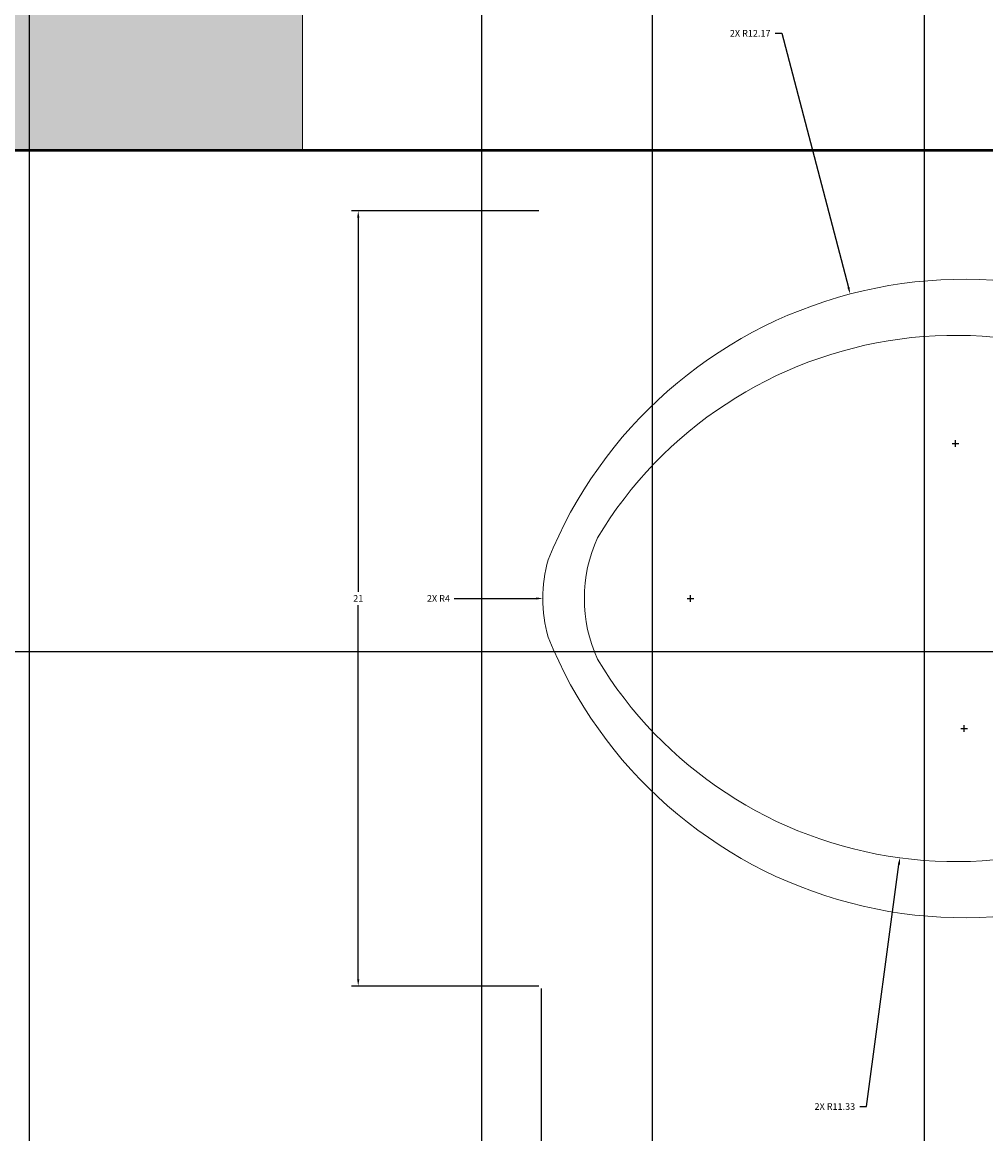
# Model space of a CAD drawing. Units: inches. Extents: x 2231 to 2461, y 2045 to 2455.
# Tile 90 of 95: x 2384 to 2410, y 2400 to 2430. Entities that reach past the tile are written whole.
import ezdxf

# ---------------------------------------------------------------- set-up
doc = ezdxf.new("R2010")
doc.units = ezdxf.units.IN
for name, color, linetype, lineweight in [('A-ANNO-DIMS', 2, 'Continuous', 18), ('A-FLOR-FIXT', 9, 'Continuous', 18), ('A-GLAZ', 4, 'Continuous', 18), ('A-WALL', 7, 'Continuous', 50)]:
    doc.layers.add(name, color=color, linetype=linetype, lineweight=lineweight)
doc.layers.add('A-WALL-PATT', color=18, linetype='Continuous', lineweight=13, true_color=0x000000)
doc.styles.get("Standard").update_dxf_attribs({"font": 'arial.ttf'})
doc.dimstyles.get("Standard").update_dxf_attribs({"dimtxt": 0.18, "dimasz": 0.18, "dimexe": 0.18, "dimexo": 0.0625, "dimgap": 0.09, "dimtad": 0, "dimtih": 1, "dimtoh": 1, "dimdec": 4, "dimzin": 0, "dimdsep": 46, "dimtxsty": 'Standard', "dimcen": 0.09, "dimadec": 0, "dimazin": 0, "dimtfac": 1, "dimtdec": 4, "dimtofl": 0, "dimtmove": 0, "dimatfit": 3, "dimfxl": 1, "dimtolj": 1, "dimtzin": 0, "dimarcsym": 0})

# ---------------------------------------------------------------- blocks, each defined once
blk = doc.blocks.new('Toilet - top')
for centre, radius, start, end in [((3.52, -21.58), 12.169, 141.4691, 247.9714), ((4.2, -21.817), 11.329, 136.3677, 238.9468), ((-3.519, -21.58), 12.169, 292.0284, 38.5307), ((-4.2, -21.817), 11.329, 301.053, 43.6321), ((0, -27.876), 4, 245.7318, 294.2682), ((0, -29), 4, 254.8605, 285.1395)]:
    blk.add_arc(centre, radius, start, end)
blk = doc.blocks.new('*D21')
at = {"layer": 'A-ANNO-DIMS', "color": 0, "lineweight": -2, "transparency": 16777216}
for p, q in [((2398.404, 2404.126), (2398.404, 2399.052)), ((2431.45, 2404.126), (2431.45, 2399.052)), ((2398.584, 2399.232), (2414.46, 2399.232)), ((2431.27, 2399.232), (2415.394, 2399.232))]:
    blk.add_line(p, q, dxfattribs=at)
at = {"layer": 'A-ANNO-DIMS', "color": 0, "transparency": 16777216}
for points in [[(2398.584, 2399.262), (2398.584, 2399.202), (2398.404, 2399.232)], [(2431.27, 2399.262), (2431.27, 2399.202), (2431.45, 2399.232)]]:
    blk.add_solid(points, dxfattribs=at)
at = {"layer": 'Defpoints', "color": 0, "transparency": 16777216}
for p in [(2398.404, 2404.189), (2431.45, 2404.189), (2431.45, 2399.232)]:
    blk.add_point(p, dxfattribs=at)
at = {"layer": 'A-ANNO-DIMS', "color": 0, "transparency": 16777216, "insert": (2414.927, 2399.232), "char_height": 0.18, "attachment_point": 5}
blk.add_mtext('\\A1;WC 33', dxfattribs=at)
blk = doc.blocks.new('*D22')
at = {"layer": 'A-ANNO-DIMS', "color": 0, "lineweight": -2, "transparency": 16777216}
for p, q in [((2398.342, 2425.189), (2393.267, 2425.189)), ((2393.447, 2425.009), (2393.447, 2414.869)), ((2393.447, 2404.369), (2393.447, 2414.508)), ((2398.342, 2404.189), (2393.267, 2404.189))]:
    blk.add_line(p, q, dxfattribs=at)
at = {"layer": 'A-ANNO-DIMS', "color": 0, "transparency": 16777216}
for points in [[(2393.417, 2425.009), (2393.477, 2425.009), (2393.447, 2425.189)], [(2393.417, 2404.369), (2393.477, 2404.369), (2393.447, 2404.189)]]:
    blk.add_solid(points, dxfattribs=at)
at = {"layer": 'Defpoints', "color": 0, "transparency": 16777216}
for p in [(2398.404, 2425.189), (2393.447, 2404.189), (2398.404, 2404.189)]:
    blk.add_point(p, dxfattribs=at)
at = {"layer": 'A-ANNO-DIMS', "color": 0, "transparency": 16777216, "insert": (2393.447, 2414.689), "char_height": 0.18, "attachment_point": 5}
blk.add_mtext('\\A1;21', dxfattribs=at)
blk = doc.blocks.new('*D36')
at = {"layer": 'A-ANNO-DIMS', "color": 0, "lineweight": -2, "transparency": 16777216}
for p, q in [((2372.794, 2426.895), (2372.794, 2454.645)), ((2372.974, 2454.465), (2402.574, 2454.465)), ((2432.614, 2454.465), (2403.013, 2454.465)), ((2432.794, 2426.895), (2432.794, 2454.645))]:
    blk.add_line(p, q, dxfattribs=at)
at = {"layer": 'A-ANNO-DIMS', "color": 0, "transparency": 16777216}
for points in [[(2372.974, 2454.495), (2372.974, 2454.435), (2372.794, 2454.465)], [(2432.614, 2454.495), (2432.614, 2454.435), (2432.794, 2454.465)]]:
    blk.add_solid(points, dxfattribs=at)
at = {"layer": 'Defpoints', "color": 0, "transparency": 16777216}
for p in [(2432.794, 2454.465), (2372.794, 2426.833), (2432.794, 2426.833)]:
    blk.add_point(p, dxfattribs=at)
at = {"layer": 'A-ANNO-DIMS', "color": 0, "transparency": 16777216, "insert": (2402.794, 2454.465), "char_height": 0.18, "attachment_point": 5}
blk.add_mtext('\\A1;60', dxfattribs=at)
blk = doc.blocks.new('*D42')
at = {"layer": 'A-ANNO-DIMS', "color": 0, "lineweight": -2, "transparency": 16777216}
for p, q in [((2396.794, 2286.895), (2396.794, 2454.645)), ((2396.974, 2454.465), (2414.575, 2454.465)), ((2432.614, 2454.465), (2415.012, 2454.465)), ((2432.794, 2286.895), (2432.794, 2454.645))]:
    blk.add_line(p, q, dxfattribs=at)
at = {"layer": 'A-ANNO-DIMS', "color": 0, "transparency": 16777216}
for points in [[(2396.974, 2454.495), (2396.974, 2454.435), (2396.794, 2454.465)], [(2432.614, 2454.495), (2432.614, 2454.435), (2432.794, 2454.465)]]:
    blk.add_solid(points, dxfattribs=at)
at = {"layer": 'Defpoints', "color": 0, "transparency": 16777216}
for p in [(2432.794, 2454.465), (2396.794, 2286.833), (2432.794, 2286.833)]:
    blk.add_point(p, dxfattribs=at)
at = {"layer": 'A-ANNO-DIMS', "color": 0, "transparency": 16777216, "insert": (2414.794, 2454.465), "char_height": 0.18, "attachment_point": 5}
blk.add_mtext('\\A1;36', dxfattribs=at)
blk = doc.blocks.new('*D59')
at = {"layer": 'A-ANNO-DIMS', "color": 0, "lineweight": -2, "transparency": 16777216}
for p, q in [((2408.794, 2182.895), (2408.794, 2454.645)), ((2408.974, 2454.465), (2420.573, 2454.465)), ((2432.614, 2454.465), (2421.014, 2454.465)), ((2432.794, 2182.895), (2432.794, 2454.645))]:
    blk.add_line(p, q, dxfattribs=at)
at = {"layer": 'A-ANNO-DIMS', "color": 0, "transparency": 16777216}
for points in [[(2408.974, 2454.495), (2408.974, 2454.435), (2408.794, 2454.465)], [(2432.614, 2454.495), (2432.614, 2454.435), (2432.794, 2454.465)]]:
    blk.add_solid(points, dxfattribs=at)
at = {"layer": 'Defpoints', "color": 0, "transparency": 16777216}
for p in [(2432.794, 2454.465), (2408.794, 2182.833), (2432.794, 2182.833)]:
    blk.add_point(p, dxfattribs=at)
at = {"layer": 'A-ANNO-DIMS', "color": 0, "transparency": 16777216, "insert": (2420.794, 2454.465), "char_height": 0.18, "attachment_point": 5}
blk.add_mtext('\\A1;24', dxfattribs=at)
blk = doc.blocks.new('*D66')
at = {"layer": 'A-ANNO-DIMS', "color": 0, "lineweight": -2, "transparency": 16777216}
for p, q in [((2348.189, 2096.895), (2348.189, 2454.645)), ((2348.369, 2454.465), (2378.167, 2454.465)), ((2408.614, 2454.465), (2378.815, 2454.465)), ((2408.794, 2096.895), (2408.794, 2454.645))]:
    blk.add_line(p, q, dxfattribs=at)
at = {"layer": 'A-ANNO-DIMS', "color": 0, "transparency": 16777216}
for points in [[(2348.369, 2454.495), (2348.369, 2454.435), (2348.189, 2454.465)], [(2408.614, 2454.495), (2408.614, 2454.435), (2408.794, 2454.465)]]:
    blk.add_solid(points, dxfattribs=at)
at = {"layer": 'Defpoints', "color": 0, "transparency": 16777216}
for p in [(2408.794, 2454.465), (2348.189, 2096.833), (2408.794, 2096.833)]:
    blk.add_point(p, dxfattribs=at)
at = {"layer": 'A-ANNO-DIMS', "color": 0, "transparency": 16777216, "insert": (2378.491, 2454.465), "char_height": 0.18, "attachment_point": 5}
blk.add_mtext('\\A1;60.6', dxfattribs=at)
blk = doc.blocks.new('*D68')
at = {"layer": 'A-ANNO-DIMS', "color": 0, "lineweight": -2, "transparency": 16777216}
for p, q in [((2285.882, 2426.833), (2460.606, 2426.833)), ((2460.426, 2426.653), (2460.426, 2420.225)), ((2460.426, 2413.433), (2460.426, 2419.861)), ((2278.251, 2413.253), (2460.606, 2413.253))]:
    blk.add_line(p, q, dxfattribs=at)
at = {"layer": 'A-ANNO-DIMS', "color": 0, "transparency": 16777216}
for points in [[(2460.396, 2426.653), (2460.456, 2426.653), (2460.426, 2426.833)], [(2460.396, 2413.433), (2460.456, 2413.433), (2460.426, 2413.253)]]:
    blk.add_solid(points, dxfattribs=at)
at = {"layer": 'Defpoints', "color": 0, "transparency": 16777216}
for p in [(2285.82, 2426.833), (2460.426, 2426.833), (2278.188, 2413.253)]:
    blk.add_point(p, dxfattribs=at)
at = {"layer": 'A-ANNO-DIMS', "color": 0, "transparency": 16777216, "insert": (2460.426, 2420.043), "char_height": 0.18, "attachment_point": 5}
blk.add_mtext('\\A1;13.58', dxfattribs=at)
blk = doc.blocks.new('*D71')
at = {"layer": 'A-ANNO-DIMS', "color": 0, "lineweight": -2, "transparency": 16777216}
for p, q in [((2401.422, 2092.979), (2401.422, 2454.645)), ((2401.602, 2454.465), (2404.732, 2454.465)), ((2408.614, 2454.465), (2405.483, 2454.465)), ((2408.794, 2096.895), (2408.794, 2454.645))]:
    blk.add_line(p, q, dxfattribs=at)
at = {"layer": 'A-ANNO-DIMS', "color": 0, "transparency": 16777216}
for points in [[(2401.602, 2454.495), (2401.602, 2454.435), (2401.422, 2454.465)], [(2408.614, 2454.495), (2408.614, 2454.435), (2408.794, 2454.465)]]:
    blk.add_solid(points, dxfattribs=at)
at = {"layer": 'Defpoints', "color": 0, "transparency": 16777216}
for p in [(2408.794, 2454.465), (2408.794, 2096.833), (2401.422, 2092.917)]:
    blk.add_point(p, dxfattribs=at)
at = {"layer": 'A-ANNO-DIMS', "color": 0, "transparency": 16777216, "insert": (2405.108, 2454.465), "char_height": 0.18, "attachment_point": 5}
blk.add_mtext('\\A1;7.371', dxfattribs=at)
blk = doc.blocks.new('*D72')
at = {"layer": 'A-ANNO-DIMS', "color": 0, "lineweight": -2, "transparency": 16777216}
for p, q in [((2384.543, 2145.12), (2384.543, 2454.645)), ((2384.723, 2454.465), (2396.272, 2454.465)), ((2408.614, 2454.465), (2397.064, 2454.465)), ((2408.794, 2150.677), (2408.794, 2454.645))]:
    blk.add_line(p, q, dxfattribs=at)
at = {"layer": 'A-ANNO-DIMS', "color": 0, "transparency": 16777216}
for points in [[(2384.723, 2454.495), (2384.723, 2454.435), (2384.543, 2454.465)], [(2408.614, 2454.495), (2408.614, 2454.435), (2408.794, 2454.465)]]:
    blk.add_solid(points, dxfattribs=at)
at = {"layer": 'Defpoints', "color": 0, "transparency": 16777216}
for p in [(2408.794, 2454.465), (2408.794, 2150.615), (2384.543, 2145.058)]:
    blk.add_point(p, dxfattribs=at)
at = {"layer": 'A-ANNO-DIMS', "color": 0, "transparency": 16777216, "insert": (2396.668, 2454.465), "char_height": 0.18, "attachment_point": 5}
blk.add_mtext('\\A1;24.25', dxfattribs=at)
blk = doc.blocks.new('*D79')
at = {"layer": 'A-ANNO-DIMS', "color": 0, "lineweight": -2, "transparency": 16777216}
for p, q in [((2404.743, 2430.001), (2404.923, 2430.001)), ((2404.923, 2430.001), (2406.732, 2423.113)), ((2409.78, 2411.169), (2409.96, 2411.169)), ((2409.87, 2411.079), (2409.87, 2411.259))]:
    blk.add_line(p, q, dxfattribs=at)
at = {"layer": 'A-ANNO-DIMS', "color": 0, "transparency": 16777216}
blk.add_solid([(2406.761, 2423.121), (2406.703, 2423.105), (2406.778, 2422.939)], dxfattribs=at)
at = {"layer": 'Defpoints', "color": 0, "transparency": 16777216}
for p in [(2406.778, 2422.939), (2409.87, 2411.169)]:
    blk.add_point(p, dxfattribs=at)
at = {"layer": 'A-ANNO-DIMS', "color": 0, "transparency": 16777216, "insert": (2404.068, 2430.001), "char_height": 0.18, "attachment_point": 5}
blk.add_mtext('\\A1;2X R12.17', dxfattribs=at)
blk = doc.blocks.new('*D80')
at = {"layer": 'A-ANNO-DIMS', "color": 0, "lineweight": -2, "transparency": 16777216}
for p, q in [((2409.543, 2418.889), (2409.723, 2418.889)), ((2409.633, 2418.799), (2409.633, 2418.979)), ((2407.217, 2400.924), (2408.099, 2407.482)), ((2407.037, 2400.924), (2407.217, 2400.924))]:
    blk.add_line(p, q, dxfattribs=at)
at = {"layer": 'A-ANNO-DIMS', "color": 0, "transparency": 16777216}
blk.add_solid([(2408.069, 2407.486), (2408.129, 2407.478), (2408.123, 2407.661)], dxfattribs=at)
at = {"layer": 'Defpoints', "color": 0, "transparency": 16777216}
for p in [(2409.633, 2418.889), (2408.123, 2407.661)]:
    blk.add_point(p, dxfattribs=at)
at = {"layer": 'A-ANNO-DIMS', "color": 0, "transparency": 16777216, "insert": (2406.362, 2400.924), "char_height": 0.18, "attachment_point": 5}
blk.add_mtext('\\A1;2X R11.33', dxfattribs=at)
blk = doc.blocks.new('*D81')
at = {"layer": 'A-ANNO-DIMS', "color": 0, "lineweight": -2, "transparency": 16777216}
for p, q in [((2396.051, 2414.689), (2398.271, 2414.689)), ((2402.361, 2414.689), (2402.541, 2414.689)), ((2402.451, 2414.599), (2402.451, 2414.779))]:
    blk.add_line(p, q, dxfattribs=at)
at = {"layer": 'A-ANNO-DIMS', "color": 0, "transparency": 16777216}
blk.add_solid([(2398.271, 2414.719), (2398.271, 2414.659), (2398.451, 2414.689)], dxfattribs=at)
at = {"layer": 'Defpoints', "color": 0, "transparency": 16777216}
for p in [(2398.451, 2414.689), (2402.451, 2414.689)]:
    blk.add_point(p, dxfattribs=at)
at = {"layer": 'A-ANNO-DIMS', "color": 0, "transparency": 16777216, "insert": (2395.621, 2414.689), "char_height": 0.18, "attachment_point": 5}
blk.add_mtext('\\A1;2X R4', dxfattribs=at)

msp = doc.modelspace()

# ---------------------------------------------------------------- hatches: boundary and pattern name
at = {"layer": 'A-WALL-PATT'}
h = msp.add_hatch(color=256, dxfattribs=at)
h.dxf.hatch_style = 1
h.paths.add_polyline_path([(2441.7935, 2269.1535), (2432.7935, 2269.1535), (2432.7935, 2186.8328), (2396.7935, 2186.8328), (2396.7935, 2286.8328), (2394.7935, 2286.8328), (2394.7935, 2186.8328), (2334.7935, 2186.8328), (2334.7935, 2182.8328), (2432.7935, 2182.8328), (2432.7935, 2072.8328), (2416.6639, 2072.8328), (2416.6639, 2063.8328), (2441.7935, 2063.8328)])
h.paths.add_polyline_path([(2368.6639, 2072.8328), (2367.04, 2072.8328), (2330.7942, 2072.8328), (2330.7397, 2063.8328), (2368.6639, 2063.8328)])
h.paths.add_polyline_path([(2300.7392, 2068.3328), (2300.7392, 2072.8328), (2298.7935, 2072.8328), (2294.7935, 2072.8328), (2258.7935, 2072.8328), (2258.7935, 2120.8328), (2294.7935, 2120.8328), (2298.7935, 2120.8328), (2298.7935, 2128.8328), (2294.7935, 2128.8328), (2294.7935, 2124.8328), (2258.7935, 2124.8328), (2258.7935, 2182.8328), (2294.7935, 2182.8328), (2294.7935, 2174.8328), (2298.7935, 2174.8328), (2298.7935, 2182.8328), (2304.7935, 2182.8328), (2304.7935, 2186.8328), (2258.7935, 2186.8328), (2258.7935, 2221.999), (2249.7935, 2221.999), (2249.7935, 2063.8328), (2300.7392, 2063.8328)])
h.paths.add_polyline_path([(2391.9338, 2435.8328), (2333.82, 2435.8328), (2333.82, 2426.8328), (2368.7935, 2426.8328), (2368.7935, 2374.9508), (2368.7935, 2370.8328), (2372.3935, 2370.8328), (2372.7935, 2370.8328), (2372.7935, 2426.8328), (2391.9338, 2426.8328)])
h.paths.add_polyline_path([(2441.7935, 2435.8328), (2415.9338, 2435.8328), (2415.9338, 2426.8328), (2432.7935, 2426.8328), (2432.7935, 2334.8328), (2372.7935, 2334.8328), (2372.7935, 2346.8328), (2368.7935, 2346.8328), (2368.7935, 2306.8328), (2360.7935, 2306.8328), (2360.7935, 2302.8328), (2368.7935, 2302.8328), (2372.7935, 2302.8328), (2372.7935, 2330.8328), (2432.7935, 2330.8328), (2432.7935, 2317.1535), (2441.7935, 2317.1535)])
h.paths.add_polyline_path([(2285.82, 2435.8328), (2249.7935, 2435.8328), (2249.7935, 2269.999), (2258.7935, 2269.999), (2258.7935, 2302.8328), (2318.8168, 2302.8328), (2330.7935, 2302.8328), (2330.7935, 2306.8328), (2258.7935, 2306.8328), (2258.7935, 2426.8328), (2285.82, 2426.8328)])

# ---------------------------------------------------------------- linework, layer by layer
at = {"layer": 'A-GLAZ'}
msp.add_line((2391.9338, 2426.8328), (2391.9338, 2435.8328), dxfattribs=at)
at = {"layer": 'A-WALL'}
msp.add_line((2372.7935, 2426.8328), (2432.7935, 2426.8328), dxfattribs=at)

# ---------------------------------------------------------------- block references
at = {"layer": 'A-FLOR-FIXT', "rotation": 270}
msp.add_blockref('Toilet - top', (2431.4505, 2414.6888), dxfattribs=at)

# ---------------------------------------------------------------- dimensions: what is measured, and where the dimension line sits
at = {"layer": 'A-ANNO-DIMS'}
for base, p1, p2, override, picture, middle in [((2408.7935, 2454.4653), (2348.1888, 2096.8328), (2408.7935, 2096.8328), {"dimdec": 1, "dimlfac": 1, "dimrnd": 0, "dimzin": 0, "dimdsep": 46, "dimlunit": 2}, '*D66', (2378.4912, 2454.4653)), ((2432.7935, 2454.4653), (2372.7935, 2426.8328), (2432.7935, 2426.8328), {"dimdec": 0, "dimlfac": 1, "dimrnd": 0, "dimzin": 0, "dimdsep": 46, "dimlunit": 2}, '*D36', (2402.7935, 2454.4653)), ((2408.7935, 2454.4653), (2384.5428, 2145.0576), (2408.7935, 2150.6145), {"dimdec": 2, "dimlfac": 1, "dimrnd": 0, "dimzin": 0, "dimdsep": 46, "dimlunit": 2}, '*D72', (2396.6682, 2454.4653)), ((2432.7935, 2454.4653), (2396.7935, 2286.8328), (2432.7935, 2286.8328), {"dimdec": 0, "dimlfac": 1, "dimrnd": 0, "dimzin": 0, "dimdsep": 46, "dimlunit": 2}, '*D42', (2414.7935, 2454.4653)), ((2408.7935, 2454.4653), (2401.4221, 2092.9167), (2408.7935, 2096.8328), {"dimdec": 3, "dimlfac": 1, "dimrnd": 0, "dimzin": 0, "dimdsep": 46, "dimlunit": 2}, '*D71', (2405.1078, 2454.4653)), ((2432.7935, 2454.4653), (2408.7935, 2182.8328), (2432.7935, 2182.8328), {"dimdec": 0, "dimlfac": 1, "dimrnd": 0, "dimzin": 0, "dimdsep": 46, "dimlunit": 2}, '*D59', (2420.7935, 2454.4653))]:
    dim = msp.add_linear_dim(base=base, p1=p1, p2=p2, dimstyle='Standard', override=override, dxfattribs=at)
    dim.commit()
    dim.dimension.update_dxf_attribs({"geometry": picture, "text_midpoint": middle})
for center, mpoint, override, picture, middle in [((2409.87, 2411.1692), (2406.778, 2422.9389), {"dimdec": 2, "dimlfac": 1, "dimrnd": 0, "dimzin": 0, "dimdsep": 46, "dimlunit": 2}, '*D79', (2404.0681, 2430.0007)), ((2409.6331, 2418.8887), (2408.1229, 2407.6606), {"dimdec": 2, "dimlfac": 1, "dimrnd": 0, "dimzin": 0, "dimdsep": 46, "dimlunit": 2}, '*D80', (2406.3621, 2400.9238)), ((2402.4505, 2414.6888), (2398.4505, 2414.689), {"dimdec": 0, "dimlfac": 1, "dimrnd": 0, "dimzin": 0, "dimdsep": 46, "dimlunit": 2}, '*D81', (2396.0505, 2414.6891))]:
    dim = msp.add_radius_dim(center=center, mpoint=mpoint, text='2X <>', dimstyle='Standard', override=override, dxfattribs=at)
    dim.commit()
    dim.dimension.update_dxf_attribs({"geometry": picture, "text_midpoint": middle, "dimtype": 164})
for base, p1, p2, angle, override, picture, middle in [((2460.426, 2426.8328), (2278.1881, 2413.2534), (2285.82, 2426.8328), 90, {"dimdec": 2, "dimlfac": 1, "dimrnd": 0, "dimzin": 0, "dimdsep": 46, "dimlunit": 2}, '*D68', (2460.426, 2420.0431)), ((2393.4473, 2404.1888), (2398.4042, 2425.1888), (2398.4042, 2404.1888), 270, {"dimdec": 0, "dimlfac": 1, "dimrnd": 0, "dimzin": 0, "dimdsep": 46, "dimlunit": 2}, '*D22', (2393.4473, 2414.6888))]:
    dim = msp.add_linear_dim(base=base, p1=p1, p2=p2, angle=angle, dimstyle='Standard', override=override, dxfattribs=at)
    dim.commit()
    dim.dimension.update_dxf_attribs({"geometry": picture, "text_midpoint": middle})
dim = msp.add_linear_dim(base=(2431.4505, 2399.2319), p1=(2398.4042, 2404.1888), p2=(2431.4505, 2404.1888), text='WC <>', dimstyle='Standard', override={"dimdec": 0, "dimlfac": 1, "dimrnd": 0, "dimzin": 0, "dimdsep": 46, "dimlunit": 2}, dxfattribs=at)
dim.commit()
dim.dimension.update_dxf_attribs({"geometry": '*D21', "text_midpoint": (2414.9274, 2399.2319)})

doc.saveas('drawing.dxf')
